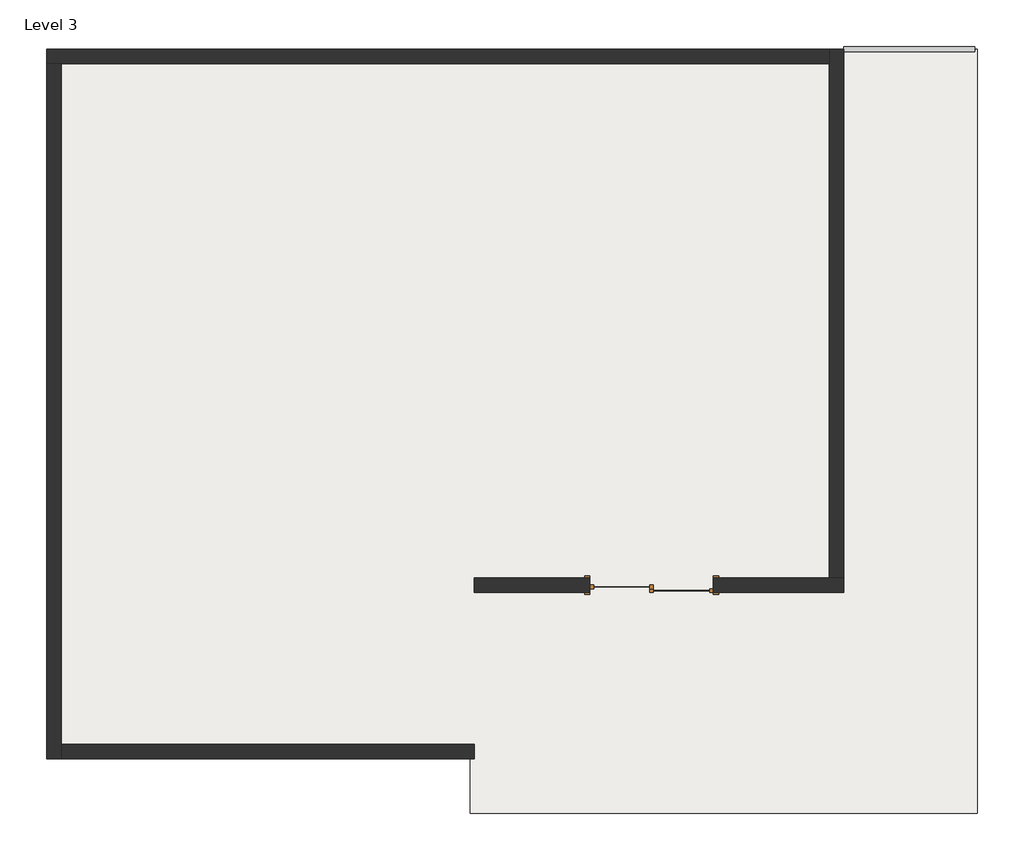
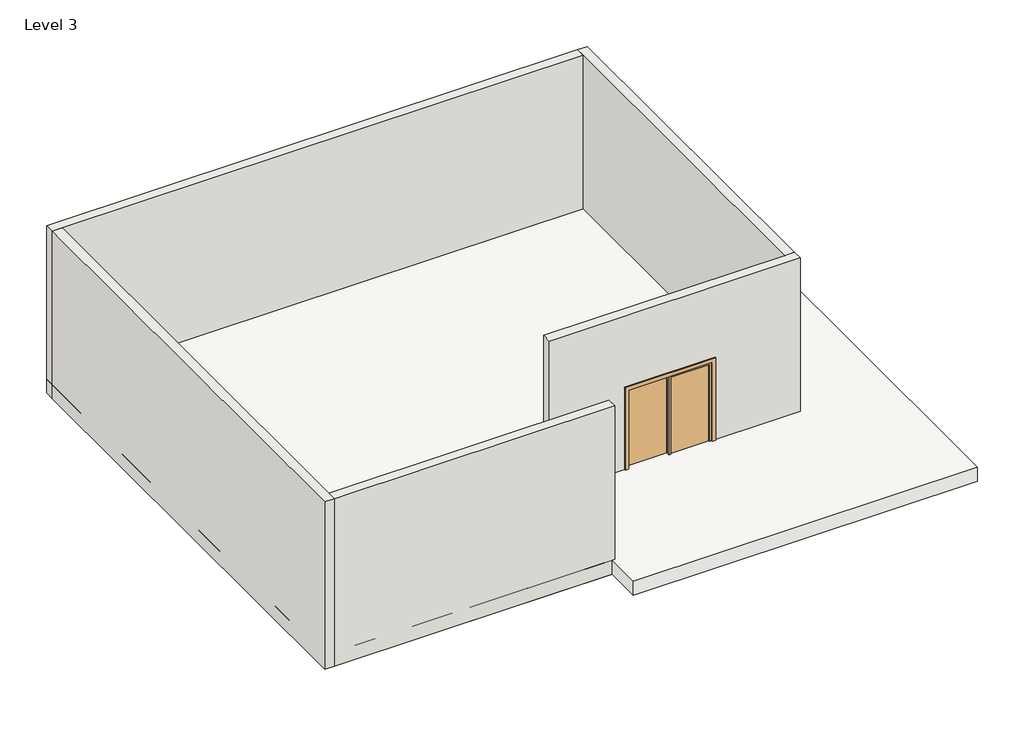
# One storey, incomplete: 5 walls, 1 door, 1 railing, 1 roof.
"""IFC4 building model written with IfcOpenShell, lengths in millimetres."""

from ifc_helpers import new_model, si_unit, point, frame, origin, place, context, project, spatial, polyline, ellipse_curve, trimmed, outline, extrude, faceted_brep, transform, mapped, element, save
from ifc_brep_helpers import plane_surface, extruded_surface, advanced_brep
from components import door_076b30e0

model = new_model("IFC4")

# Units and contexts
model_context = context("Model", 3, world=origin())
ifc_project = project(units=[si_unit("LENGTHUNIT", "METRE", prefix="MILLI")], contexts=[model_context])

# Site, building, storey
site = spatial("IfcSite", under=ifc_project)
building = spatial("IfcBuilding", under=site)
storey = spatial("IfcBuildingStorey", under=building, Name="Level 3", Elevation=7315.2)

# Door
placement = place(None, origin())
door_shape = door_076b30e0(model_context)
element("IfcDoor", 1, ObjectType="Door-Double-Sliding : 68\" x 80\"", at=placement, inside=storey, context=model_context, shape_type="MappedRepresentation", body=[
    mapped(door_shape, transform((-2468.3371298, 3709.9359817, 7315.2), x_axis=(-1.0, 0.0, 0.0), y_axis=(0.0, -1.0, 0.0), z_axis=(0.0, 0.0, 1.0))),
])

# Railing
element("IfcRailing", 2, ObjectType="Glass Panel - Bottom Fill", at=placement, inside=storey, context=model_context, shape_type="SolidModel", body=[
    advanced_brep(
    [(2062.5612535, 11063.2359817, 8229.6), (2062.5612535, 11139.4359817, 8229.6), (224.0628702, 11063.2359817, 8229.6), (224.0628702, 11139.4359817, 8229.6)],
    [
        (0, 1, ellipse_curve(frame((2062.5612535, 11101.3359817, 8229.6), z_axis=(1.0, 0.0, 0.0), x_axis=(0.0, 1.0, 0.0)), 38.1, 28.575)),
        (1, 0, ellipse_curve(frame((2062.5612535, 11101.3359817, 8229.6), z_axis=(1.0, 0.0, 0.0), x_axis=(0.0, 1.0, 0.0)), 38.1, 28.575)),
        (2, 3, ellipse_curve(frame((224.0628702, 11101.3359817, 8229.6), z_axis=(-1.0, 0.0, 0.0), x_axis=(0.0, 1.0, 0.0)), 38.1, 28.575)),
        (3, 2, ellipse_curve(frame((224.0628702, 11101.3359817, 8229.6), z_axis=(-1.0, 0.0, 0.0), x_axis=(0.0, 1.0, 0.0)), 38.1, 28.575)),
        (0, 2),
        (3, 1),
    ],
    [
        plane_surface(frame((2062.5612535, 11101.3359817, 8229.6), z_axis=(1.0, 0.0, 0.0), x_axis=(0.0, -1.0, 0.0))),
        plane_surface(frame((224.0628702, 11101.3359817, 8229.6), z_axis=(-1.0, 0.0, 0.0), x_axis=(0.0, -1.0, 0.0))),
        extruded_surface(trimmed(ellipse_curve(frame((224.0628702, 11101.3359817, 8229.6), z_axis=(1.0, 0.0, 0.0), x_axis=(0.0, 1.0, 0.0)), 38.1, 28.575), [point((224.0628702, 11063.2359817, 8229.6))], [point((224.0628702, 11139.4359817, 8229.6))], True, "CARTESIAN"), (1838.4983833000001, 0.0, 0.0), 1838.4983833000001),
        extruded_surface(trimmed(ellipse_curve(frame((224.0628702, 11101.3359817, 8229.6), z_axis=(1.0, 0.0, 0.0), x_axis=(0.0, 1.0, 0.0)), 38.1, 28.575), [point((224.0628702, 11139.4359817, 8229.6))], [point((224.0628702, 11063.2359817, 8229.6))], True, "CARTESIAN"), (1838.4983833000001, 0.0, 0.0), 1838.4983833000001),
    ],
    [
        (0, [[1, 2]]),
        (1, [[3, 4]]),
        (2, [[-1, 5, -4, 6]]),
        (3, [[-2, -6, -3, -5]]),
    ],
),
    extrude(outline(polyline([(2062.5612535, 11114.0359817), (2062.5612535, 11088.6359817), (224.0628702, 11088.6359817), (224.0628702, 11114.0359817), (2062.5612535, 11114.0359817)])), frame((0.0, 0.0, 8115.3), z_axis=(0.0, 0.0, 1.0), x_axis=(1.0, 0.0, 0.0)), (0.0, 0.0, 1.0), 25.4),
    extrude(outline(polyline([(2062.5612535, 11114.0359817), (2062.5612535, 11088.6359817), (224.0628702, 11088.6359817), (224.0628702, 11114.0359817), (2062.5612535, 11114.0359817)])), frame((0.0, 0.0, 8013.7), z_axis=(0.0, 0.0, 1.0), x_axis=(1.0, 0.0, 0.0)), (0.0, 0.0, 1.0), 25.4),
    extrude(outline(polyline([(336.8620618, 11126.7359817), (336.8620618, 11075.9359817), (324.1620618, 11075.9359817), (324.1620618, 11126.7359817), (336.8620618, 11126.7359817)])), frame((0.0, 0.0, 7315.2), z_axis=(0.0, 0.0, 1.0), x_axis=(1.0, 0.0, 0.0)), (0.0, 0.0, 1.0), 885.6788223),
    extrude(outline(polyline([(1143.3120618, 11094.8008247), (330.5120618, 11094.8008247), (330.5120618, 11101.1508247), (1143.3120618, 11101.1508247), (1143.3120618, 11094.8008247)])), frame((0.0, 0.0, 7416.8), z_axis=(0.0, 0.0, 1.0), x_axis=(1.0, 0.0, 0.0)), (0.0, 0.0, 1.0), 596.9),
    extrude(outline(polyline([(1149.6620618, 11126.7359817), (1149.6620618, 11075.9359817), (1136.9620618, 11075.9359817), (1136.9620618, 11126.7359817), (1149.6620618, 11126.7359817)])), frame((0.0, 0.0, 7315.2), z_axis=(0.0, 0.0, 1.0), x_axis=(1.0, 0.0, 0.0)), (0.0, 0.0, 1.0), 885.6788223),
    extrude(outline(polyline([(1956.1120618, 11094.8008247), (1143.3120618, 11094.8008247), (1143.3120618, 11101.1508247), (1956.1120618, 11101.1508247), (1956.1120618, 11094.8008247)])), frame((0.0, 0.0, 7416.8), z_axis=(0.0, 0.0, 1.0), x_axis=(1.0, 0.0, 0.0)), (0.0, 0.0, 1.0), 596.9),
    extrude(outline(polyline([(1962.4620618, 11126.7359817), (1962.4620618, 11075.9359817), (1949.7620618, 11075.9359817), (1949.7620618, 11126.7359817), (1962.4620618, 11126.7359817)])), frame((0.0, 0.0, 7315.2), z_axis=(0.0, 0.0, 1.0), x_axis=(1.0, 0.0, 0.0)), (0.0, 0.0, 1.0), 885.6788223),
    extrude(outline(polyline([(236.7628702, 11110.8609817), (236.7628702, 11091.8109817), (217.7128702, 11091.8109817), (217.7128702, 11110.8609817), (236.7628702, 11110.8609817)])), frame((0.0, 0.0, 7315.2), z_axis=(0.0, 0.0, 1.0), x_axis=(1.0, 0.0, 0.0)), (0.0, 0.0, 1.0), 885.6788223),
    extrude(outline(polyline([(2068.9112535, 11110.8609817), (2068.9112535, 11091.8109817), (2049.8612535, 11091.8109817), (2049.8612535, 11110.8609817), (2068.9112535, 11110.8609817)])), frame((0.0, 0.0, 7315.2), z_axis=(0.0, 0.0, 1.0), x_axis=(1.0, 0.0, 0.0)), (0.0, 0.0, 1.0), 885.6788223),
])

# Roof
element("IfcRoof", 3, ObjectType="Generic - 12\"", at=placement, inside=storey, context=model_context, shape_type="SweptSolid", body=[
    extrude(outline(polyline([(-10951.9371298, 11101.3359817), (2101.2415497, 11101.3359817), (2101.2415497, 1144.5359817), (2101.2415497, 382.5359817), (-5008.3371298, 382.5359817), (-5008.3371298, 1144.5359817), (-10951.9371298, 1144.5359817), (-10951.9371298, 11101.3359817)])), frame((0.0, 0.0, 7315.2), z_axis=(0.0, 0.0, 1.0), x_axis=(1.0, 0.0, 0.0)), (0.0, 0.0, 1.0), 304.8),
])

# Walls
element("IfcWall", 4, ObjectType="Generic - 8\"", at=placement, inside=storey, context=model_context, shape_type="Brep", body=[
    faceted_brep([(-10951.9371298, 10898.1359817, 7315.2), (-10748.7371298, 10898.1359817, 7315.2), (20.8628702, 10898.1359817, 7315.2), (20.8628702, 10898.1359817, 10972.8), (-10748.7371298, 10898.1359817, 10972.8), (-10951.9371298, 10898.1359817, 10972.8), (-10951.9371298, 11101.3359817, 7315.2), (-10951.9371298, 11101.3359817, 10972.8), (20.8628702, 11101.3359817, 10972.8), (20.8628702, 11101.3359817, 7315.2)], [[[0, 1, 2, 3, 4, 5]], [[6, 7, 8, 9]], [[2, 1, 0, 6, 9]], [[5, 4, 3, 8, 7]], [[0, 5, 7, 6]], [[3, 2, 9, 8]]]),
])
element("IfcWall", 5, ObjectType="Generic - 8\"", at=placement, inside=storey, context=model_context, shape_type="Brep", body=[
    faceted_brep([(-10748.7371298, 1144.5359817, 7315.2), (-10748.7371298, 1347.7359817, 7315.2), (-10748.7371298, 10898.1359817, 7315.2), (-10748.7371298, 10898.1359817, 10972.8), (-10748.7371298, 1347.7359817, 10972.8), (-10748.7371298, 1144.5359817, 10972.8), (-10951.9371298, 1144.5359817, 7315.2), (-10951.9371298, 1144.5359817, 10972.8), (-10951.9371298, 10898.1359817, 10972.8), (-10951.9371298, 10898.1359817, 7315.2)], [[[0, 1, 2, 3, 4, 5]], [[6, 7, 8, 9]], [[2, 1, 0, 6, 9]], [[5, 4, 3, 8, 7]], [[0, 5, 7, 6]], [[3, 2, 9, 8]]]),
])
element("IfcWall", 6, ObjectType="Generic - 8\"", at=placement, inside=storey, context=model_context, shape_type="Brep", body=[
    faceted_brep([(-4957.5371298, 1347.7359817, 7315.2), (-10748.7371298, 1347.7359817, 7315.2), (-10748.7371298, 1347.7359817, 10972.8), (-4957.5371298, 1347.7359817, 10972.8), (-4957.5371298, 1347.7359817, 9753.6), (-4957.5371298, 1144.5359817, 7315.2), (-4957.5371298, 1144.5359817, 10972.8), (-10748.7371298, 1144.5359817, 10972.8), (-10748.7371298, 1144.5359817, 7315.2)], [[[0, 1, 2, 3, 4]], [[5, 6, 7, 8]], [[1, 0, 5, 8]], [[3, 2, 7, 6]], [[2, 1, 8, 7]], [[0, 4, 3, 6, 5]]]),
])
element("IfcWall", 7, ObjectType="Generic - 8\"", at=placement, inside=storey, context=model_context, shape_type="Brep", body=[
    faceted_brep([(20.8628702, 11101.3359817, 7315.2), (20.8628702, 10898.1359817, 7315.2), (20.8628702, 3684.5359817, 7315.2), (20.8628702, 3684.5359817, 10972.8), (20.8628702, 10898.1359817, 10972.8), (20.8628702, 11101.3359817, 10972.8), (224.0628702, 11101.3359817, 7315.2), (224.0628702, 11101.3359817, 10972.8), (224.0628702, 3684.5359817, 10972.8), (224.0628702, 3684.5359817, 7315.2)], [[[0, 1, 2, 3, 4, 5]], [[6, 7, 8, 9]], [[2, 1, 0, 6, 9]], [[5, 4, 3, 8, 7]], [[0, 5, 7, 6]], [[3, 2, 9, 8]]]),
])
element("IfcWall", 8, ObjectType="Generic - 8\"", at=placement, inside=storey, context=model_context, shape_type="Brep", body=[
    faceted_brep([(-4957.5371298, 3481.3359817, 7315.2), (-3331.9371298, 3481.3359817, 7315.2), (-3331.9371298, 3481.3359817, 9347.2), (-1604.7371298, 3481.3359817, 9347.2), (-1604.7371298, 3481.3359817, 7315.2), (224.0628702, 3481.3359817, 7315.2), (224.0628702, 3481.3359817, 10972.8), (-4957.5371298, 3481.3359817, 10972.8), (-3331.9371298, 3684.5359817, 9347.2), (-3331.9371298, 3684.5359817, 7315.2), (-4957.5371298, 3684.5359817, 7315.2), (-4957.5371298, 3684.5359817, 9753.6), (-4957.5371298, 3684.5359817, 10972.8), (20.8628702, 3684.5359817, 10972.8), (224.0628702, 3684.5359817, 10972.8), (224.0628702, 3684.5359817, 7315.2), (20.8628702, 3684.5359817, 7315.2), (-1604.7371298, 3684.5359817, 7315.2), (-1604.7371298, 3684.5359817, 9347.2)], [[[0, 1, 2, 3, 4, 5, 6, 7]], [[8, 9, 10, 11, 12, 13, 14, 15, 16, 17, 18]], [[10, 9, 1, 0]], [[17, 16, 15, 5, 4]], [[7, 6, 14, 13, 12]], [[0, 7, 12, 11, 10]], [[6, 5, 15, 14]], [[4, 3, 18, 17]], [[2, 1, 9, 8]], [[3, 2, 8, 18]]]),
])

save(model, "model.ifc")

# Revit data of these elements
# Type "Door-Double-Sliding : 68\" x 80\""
#   Type Mark = "9"
#   Construction Type Id = "opn-d45"
#   Assembly Code = "C1020"
#   Analytic Construction = "Wood frame, double glass door "
#   Thickness = 0' - 2"
#   Thermal Resistance (R) = 1.8150 (h·ft²·°F)/BTU
#   Heat Transfer Coefficient (U) = 0.5510 BTU/(h·ft²·°F)
#   Height = 6' - 8"
#   Rail Width = 0' - 2"
#   Stiles = 0' - 2"
#   Trim Projection Ext = 0' - 1"
#   Trim Projection Int = 0' - 1"
#   Trim Width = 0' - 3"
#   Width = 5' - 8"
#   Define Thermal Properties by = 1
#   Glazing = Glass
#   Panel Material = Wood - Birch - Solid Stained Light Low Gloss
#   Trim Material = Paint - Sienna
#   Visual Light Transmittance = 0
#   Solar Heat Gain Coefficient = 0
#   Function = (empty or 0)
#   Wall Closure = (empty or 0)
# Type "Glass Panel - Bottom Fill"
#   Assembly Code = "C2010400"
#   built-in parameter 1008612 = 0.0416667 (stored number, unit not read)
#   built-in parameter 1008611 = 0.0416667 (stored number, unit not read)
#   built-in parameter 1008609 = 0.333333 (stored number, unit not read)
#   built-in parameter 1008604 = 0.166667 (stored number, unit not read)
#   built-in parameter 1008603 = 0.166667 (stored number, unit not read)
#   Railing Height = 3' - 0"
#   built-in parameter 1008630 = 2
#   built-in parameter 1008610 = 2
#   built-in parameter 1008618 = Baluster - Square : 3/4"
# Type "Generic - 12\""
#   Assembly Code = "B1020"
#   Layers, outside or top first: 1' - 0" no material (function 1)
# Type "Generic - 8\""
#   Assembly Code = "B2010"
#   Layers, outside or top first: 0' - 8" no material (function 1)
# Element 1 (IfcDoor, "Door-Double-Sliding : 68\" x 80\"")
#   Phase Created = New Construction
#   Materials on its faces: "Paint - Sienna", "Wood - Birch - Solid Stained Light Low Gloss", "Glass"
# Element 2 (IfcRailing, "Glass Panel - Bottom Fill")
#   Phase Created = New Construction
#   Materials on its faces: "Glass"
# Element 3 (IfcRoof, "Generic - 12\"")
#   built-in parameter 1001705 = 25 (stored number, unit not read)
#   built-in parameter 1001710 = 33615
#   Phase Created = New Construction
#   Materials on its faces: "Default Roof"
# Elements 4, 5, 6, 7, 8 (IfcWall, "Generic - 8\"")
#   Top Offset = 0' - 0"
#   Base Offset = 0' - 0"
#   Unconnected Height = 12' - 0"
#   wall height = 12' - 0"
#   Phase Created = New Construction
#   Base Constraint = Level 3
#   Materials on its faces: "Default Wall"
# Materials
#   "Glass": class "Glass", colour RGB 0 128 192, transparency 0.75, Description = "Soda Lime Glass", Cost = 0
#   "Wood - Birch - Solid Stained Light Low Gloss": class "Wood", colour RGB 210 159 95, transparency 0, Cost = 0
#   "Paint - Sienna": colour RGB 118 70 51, transparency 0, Cost = 0
#   "Default Roof": colour RGB 88 101 114, transparency 0
#   "Default Wall": colour RGB 128 128 128, transparency 0
